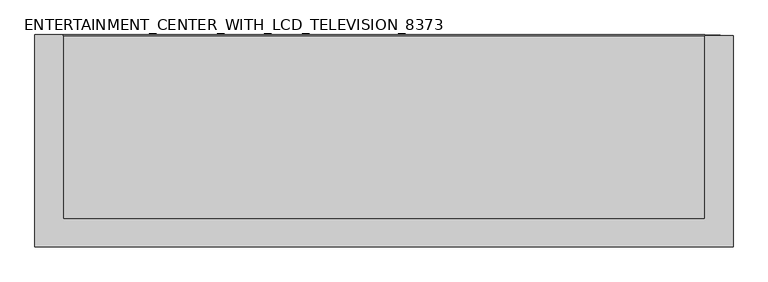
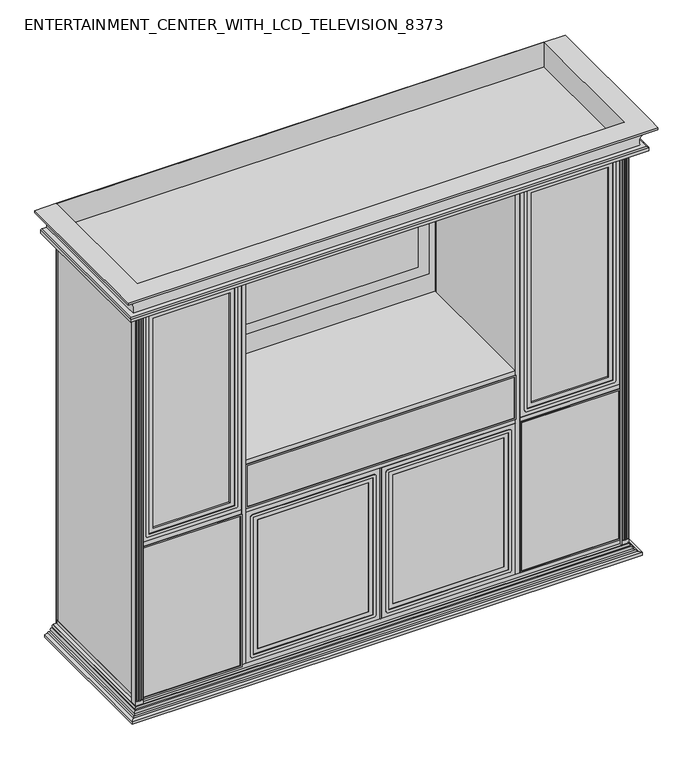
"""IFC4 building model written with IfcOpenShell, lengths in millimetres: furniture geometry, ENTERTAINMENT_CENTER_WITH_LCD_TELEVISION_8373."""

from ifc_helpers import new_model, si_unit, point, frame, frame_2d, origin, origin_with_axes, place, context, project, spatial, polyline, circle_curve, ellipse_curve, trimmed, segment, composite_curve, outline, extrude, faceted_brep, source, transform, mapped, element, save
from ifc_brep_helpers import plane_surface, cylinder_surface, revolved_surface, advanced_brep


def entertainment_center_with_lcd_television_8373_4fd72ac7(model_context):
    return source(origin(), model_context, "Body", "SolidModel", [
        extrude(outline(polyline([(-1066.8, -9.525), (-1066.8, 0.0), (-1047.75, 0.0), (-1047.75, -9.525), (-1047.75, -609.6), (-1066.8, -609.6), (-1066.8, -9.525)])), frame((0.0, 0.0, 19.05), z_axis=(0.0, 0.0, 1.0), x_axis=(1.0, 0.0, 0.0)), (0.0, 0.0, 1.0), 1790.7),
        extrude(outline(polyline([(1066.8, -9.525), (1066.8, -609.6), (1047.75, -609.6), (1047.75, -9.525), (1047.75, 0.0), (1066.8, 0.0), (1066.8, -9.525)])), frame((0.0, 0.0, 19.05), z_axis=(0.0, 0.0, 1.0), x_axis=(1.0, 0.0, 0.0)), (0.0, 0.0, 1.0), 1790.7),
        extrude(outline(polyline([(609.6, -9.525), (609.6, -609.6), (590.55, -609.6), (590.55, -9.525), (590.55, 0.0), (609.6, 0.0), (609.6, -9.525)])), frame((0.0, 0.0, 19.05), z_axis=(0.0, 0.0, 1.0), x_axis=(1.0, 0.0, 0.0)), (0.0, 0.0, 1.0), 1790.7),
        extrude(outline(polyline([(-590.55, -9.525), (-590.55, -609.6), (-609.6, -609.6), (-609.6, -9.525), (-609.6, 0.0), (-590.55, 0.0), (-590.55, -9.525)])), frame((0.0, 0.0, 19.05), z_axis=(0.0, 0.0, 1.0), x_axis=(1.0, 0.0, 0.0)), (0.0, 0.0, 1.0), 1790.7),
        extrude(outline(polyline([(590.55, -609.6), (-590.55, -609.6), (-590.55, 0.0), (590.55, 0.0), (590.55, -609.6)])), frame((0.0, 0.0, 717.55), z_axis=(0.0, 0.0, 1.0), x_axis=(1.0, 0.0, 0.0)), (0.0, 0.0, 1.0), 19.05),
        extrude(outline(polyline([(2.2792992, -609.6), (-2.4300659, -609.6), (-2.4300659, -590.55), (2.2792992, -590.55), (2.2792992, -609.6)])), frame((0.0, 0.0, 19.05), z_axis=(0.0, 0.0, 1.0), x_axis=(1.0, 0.0, 0.0)), (0.0, 0.0, 1.0), 698.5),
        extrude(outline(polyline([(717.55, -3.175), (717.55, -590.55), (19.05, -590.55), (19.05, -3.175), (717.55, -3.175)]), holes=[polyline([(666.75, -53.975), (69.85, -53.975), (69.85, -539.75), (666.75, -539.75), (666.75, -53.975)])]), frame((0.0, -609.6, 0.0), z_axis=(0.0, 1.0, 0.0), x_axis=(0.0, 0.0, 1.0)), (0.0, 0.0, 1.0), 19.05),
        extrude(outline(polyline([(717.55, 590.55), (717.55, 3.175), (19.05, 3.175), (19.05, 590.55), (717.55, 590.55)]), holes=[polyline([(666.75, 539.75), (69.85, 539.75), (69.85, 53.975), (666.75, 53.975), (666.75, 539.75)])]), frame((0.0, -609.6, 0.0), z_axis=(0.0, 1.0, 0.0), x_axis=(0.0, 0.0, 1.0)), (0.0, 0.0, 1.0), 19.05),
        extrude(outline(polyline([(-53.975, -609.6), (-539.75, -609.6), (-539.75, -606.425), (-53.975, -606.425), (-53.975, -609.6)])), frame((0.0, 0.0, 69.85), z_axis=(0.0, 0.0, 1.0), x_axis=(1.0, 0.0, 0.0)), (0.0, 0.0, 1.0), 596.9),
        extrude(outline(polyline([(539.75, -609.6), (53.975, -609.6), (53.975, -606.425), (539.75, -606.425), (539.75, -609.6)])), frame((0.0, 0.0, 69.85), z_axis=(0.0, 0.0, 1.0), x_axis=(1.0, 0.0, 0.0)), (0.0, 0.0, 1.0), 596.9),
        extrude(outline(polyline([(-609.6, -609.6), (-1047.75, -609.6), (-1047.75, 0.0), (-609.6, 0.0), (-609.6, -609.6)])), frame((0.0, 0.0, 717.55), z_axis=(0.0, 0.0, 1.0), x_axis=(1.0, 0.0, 0.0)), (0.0, 0.0, 1.0), 19.05),
        extrude(outline(polyline([(1047.75, -609.6), (609.6, -609.6), (609.6, 0.0), (1047.75, 0.0), (1047.75, -609.6)])), frame((0.0, 0.0, 717.55), z_axis=(0.0, 0.0, 1.0), x_axis=(1.0, 0.0, 0.0)), (0.0, 0.0, 1.0), 19.05),
        extrude(outline(polyline([(590.55, -609.6), (-590.55, -609.6), (-590.55, 0.0), (590.55, 0.0), (590.55, -609.6)])), frame((0.0, 0.0, 939.8), z_axis=(0.0, 0.0, 1.0), x_axis=(1.0, 0.0, 0.0)), (0.0, 0.0, 1.0), 19.05),
        extrude(outline(polyline([(590.55, -609.6), (-590.55, -609.6), (-590.55, -590.55), (590.55, -590.55), (590.55, -609.6)])), frame((0.0, 0.0, 736.6), z_axis=(0.0, 0.0, 1.0), x_axis=(1.0, 0.0, 0.0)), (0.0, 0.0, 1.0), 203.2),
        extrude(outline(polyline([(-609.6, -609.6), (-1047.75, -609.6), (-1047.75, -590.55), (-609.6, -590.55), (-609.6, -609.6)])), frame((0.0, 0.0, 19.05), z_axis=(0.0, 0.0, 1.0), x_axis=(1.0, 0.0, 0.0)), (0.0, 0.0, 1.0), 698.5),
        extrude(outline(polyline([(1047.75, -609.6), (609.6, -609.6), (609.6, -590.55), (1047.75, -590.55), (1047.75, -609.6)])), frame((0.0, 0.0, 19.05), z_axis=(0.0, 0.0, 1.0), x_axis=(1.0, 0.0, 0.0)), (0.0, 0.0, 1.0), 698.5),
        extrude(outline(polyline([(-609.6, -547.2385418), (-1047.75, -547.2385418), (-1047.75, 0.0), (-609.6, 0.0), (-609.6, -547.2385418)])), frame((0.0, 0.0, 1291.7854241), z_axis=(0.0, 0.0, 1.0), x_axis=(1.0, 0.0, 0.0)), (0.0, 0.0, 1.0), 3.175),
        extrude(outline(polyline([(1047.75, -547.2385418), (609.6, -547.2385418), (609.6, 0.0), (1047.75, 0.0), (1047.75, -547.2385418)])), frame((0.0, 0.0, 1291.7854241), z_axis=(0.0, 0.0, 1.0), x_axis=(1.0, 0.0, 0.0)), (0.0, 0.0, 1.0), 3.175),
        extrude(outline(polyline([(-609.6, -547.2385418), (-1047.75, -547.2385418), (-1047.75, 0.0), (-609.6, 0.0), (-609.6, -547.2385418)])), frame((0.0, 0.0, 887.1114077), z_axis=(0.0, 0.0, 1.0), x_axis=(1.0, 0.0, 0.0)), (0.0, 0.0, 1.0), 3.175),
        extrude(outline(polyline([(1047.75, -547.2385418), (609.6, -547.2385418), (609.6, 0.0), (1047.75, 0.0), (1047.75, -547.2385418)])), frame((0.0, 0.0, 887.1114077), z_axis=(0.0, 0.0, 1.0), x_axis=(1.0, 0.0, 0.0)), (0.0, 0.0, 1.0), 3.175),
        extrude(outline(polyline([(-609.6, -547.2385418), (-1047.75, -547.2385418), (-1047.75, 0.0), (-609.6, 0.0), (-609.6, -547.2385418)])), frame((0.0, 0.0, 1501.775), z_axis=(0.0, 0.0, 1.0), x_axis=(1.0, 0.0, 0.0)), (0.0, 0.0, 1.0), 3.175),
        extrude(outline(polyline([(1047.75, -547.2385418), (609.6, -547.2385418), (609.6, 0.0), (1047.75, 0.0), (1047.75, -547.2385418)])), frame((0.0, 0.0, 1501.775), z_axis=(0.0, 0.0, 1.0), x_axis=(1.0, 0.0, 0.0)), (0.0, 0.0, 1.0), 3.175),
        extrude(outline(polyline([(546.1, -29.8156633), (-546.1, -29.8156633), (-546.1, 0.0), (546.1, 0.0), (546.1, -29.8156633)])), frame((0.0, 0.0, 1073.15), z_axis=(0.0, 0.0, 1.0), x_axis=(1.0, 0.0, 0.0)), (0.0, 0.0, 1.0), 660.4),
        extrude(outline(polyline([(495.3, -36.468697), (-495.3, -36.468697), (-495.3, -29.8156633), (495.3, -29.8156633), (495.3, -36.468697)])), frame((0.0, 0.0, 1123.95), z_axis=(0.0, 0.0, 1.0), x_axis=(1.0, 0.0, 0.0)), (0.0, 0.0, 1.0), 558.8),
        extrude(outline(polyline([(1066.8, 3.175), (1066.8, 0.0), (-1066.8, 0.0), (-1066.8, 3.175), (1066.8, 3.175)])), origin_with_axes(), (0.0, 0.0, 1.0), 1942.4645734),
        extrude(outline(polyline([(1066.8, -609.6), (-1066.8, -609.6), (-1066.8, 0.0), (1066.8, 0.0), (1066.8, -609.6)])), origin_with_axes(), (0.0, 0.0, 1.0), 19.05),
        extrude(outline(polyline([(1066.8, -609.6), (-1066.8, -609.6), (-1066.8, 0.0), (1066.8, 0.0), (1066.8, -609.6)])), frame((0.0, 0.0, 1809.75), z_axis=(0.0, 0.0, 1.0), x_axis=(1.0, 0.0, 0.0)), (0.0, 0.0, 1.0), 19.05),
        advanced_brep(
        [(1066.8, 3.175, 0.0), (1066.8, -609.6, 0.0), (-1066.8, -609.6, 0.0), (-1066.8, 3.175, 0.0), (-1079.6325221, 3.175, 0.0), (-1079.6325221, -622.4325221, 0.0), (1079.6325221, -622.4325221, 0.0), (1079.6325221, 3.175, 0.0), (-1066.8, 3.175, -47.0950188), (-1066.8, -609.6, -47.0950188), (1066.8, -609.6, -47.0950188), (1066.8, 3.175, -47.0950188), (1117.6, 3.175, -47.0950188), (1117.6, -660.4, -47.0950188), (-1117.6, -660.4, -47.0950188), (-1117.6, 3.175, -47.0950188), (-1117.6, 3.175, -34.925), (-1103.8793251, 3.175, -32.3686785), (-1097.6139898, 3.175, -29.2621608), (-1090.9923514, 3.175, -24.0948191), (-1084.548346, 3.175, -15.7775241), (-1082.539262, 3.175, -11.7365609), (-1079.9769539, 3.175, -2.8346923), (-1117.6, -660.4, -34.925), (1117.6, -660.4, -34.925), (1117.6, 3.175, -34.925), (1079.9769539, 3.175, -2.8346923), (1082.539262, 3.175, -11.7365609), (1084.548346, 3.175, -15.7775241), (1090.9923514, 3.175, -24.0948191), (1097.6139898, 3.175, -29.2621608), (1103.8793251, 3.175, -32.3686785), (1079.9769539, -622.7769539, -2.8346923), (-1079.9769539, -622.7769539, -2.8346923), (1103.8793251, -646.6793251, -32.3686785), (1097.6139898, -640.4139898, -29.2621608), (1090.9923514, -633.7923514, -24.0948191), (1084.548346, -627.348346, -15.7775241), (1082.539262, -625.339262, -11.7365609), (-1103.8793251, -646.6793251, -32.3686785), (-1097.6139898, -640.4139898, -29.2621608), (-1090.9923514, -633.7923514, -24.0948191), (-1084.548346, -627.348346, -15.7775241), (-1082.539262, -625.339262, -11.7365609)],
        [
            (0, 1),
            (1, 2),
            (2, 3),
            (3, 4),
            (4, 5),
            (5, 6),
            (6, 7),
            (7, 0),
            (8, 9),
            (9, 10),
            (10, 11),
            (11, 12),
            (12, 13),
            (13, 14),
            (14, 15),
            (15, 8),
            (15, 16),
            (16, 17, circle_curve(frame((-1117.6, 3.175, 3.175), z_axis=(0.0, -1.0, 0.0), x_axis=(1.0, 0.0, 0.0)), 38.1)),
            (17, 18, circle_curve(frame((-1100.6752321, 3.175, -30.9594728), z_axis=(0.0, 1.0, 0.0), x_axis=(1.0, 0.0, 0.0)), 3.5002961)),
            (18, 19, circle_curve(frame((-1117.6, 3.175, 3.175), z_axis=(0.0, -1.0, 0.0), x_axis=(1.0, 0.0, 0.0)), 38.1)),
            (19, 20, circle_curve(frame((-1087.4818585, 3.175, -20.1596857), z_axis=(0.0, 1.0, 0.0), x_axis=(1.0, 0.0, 0.0)), 5.2734083)),
            (20, 21, circle_curve(frame((-1117.6, 3.175, 3.175), z_axis=(0.0, -1.0, 0.0), x_axis=(1.0, 0.0, 0.0)), 38.1)),
            (21, 22, circle_curve(frame((-1080.9865607, 3.175, -7.3637886), z_axis=(0.0, 1.0, 0.0), x_axis=(1.0, 0.0, 0.0)), 4.6402607)),
            (22, 4, circle_curve(frame((-1117.6, 3.175, 3.175), z_axis=(0.0, -1.0, 0.0), x_axis=(1.0, 0.0, 0.0)), 38.1)),
            (3, 8),
            (14, 23),
            (23, 16),
            (13, 24),
            (24, 23),
            (12, 25),
            (25, 24),
            (11, 0),
            (7, 26, circle_curve(frame((1117.6, 3.175, 3.175), z_axis=(0.0, -1.0, 0.0), x_axis=(-1.0, 0.0, 0.0)), 38.1)),
            (26, 27, circle_curve(frame((1080.9865607, 3.175, -7.3637886), z_axis=(0.0, 1.0, 0.0), x_axis=(-1.0, 0.0, 0.0)), 4.6402607)),
            (27, 28, circle_curve(frame((1117.6, 3.175, 3.175), z_axis=(0.0, -1.0, 0.0), x_axis=(-1.0, 0.0, 0.0)), 38.1)),
            (28, 29, circle_curve(frame((1087.4818585, 3.175, -20.1596857), z_axis=(0.0, 1.0, 0.0), x_axis=(-1.0, 0.0, 0.0)), 5.2734083)),
            (29, 30, circle_curve(frame((1117.6, 3.175, 3.175), z_axis=(0.0, -1.0, 0.0), x_axis=(-1.0, 0.0, 0.0)), 38.1)),
            (30, 31, circle_curve(frame((1100.6752321, 3.175, -30.9594728), z_axis=(0.0, 1.0, 0.0), x_axis=(-1.0, 0.0, 0.0)), 3.5002961)),
            (31, 25, circle_curve(frame((1117.6, 3.175, 3.175), z_axis=(0.0, -1.0, 0.0), x_axis=(-1.0, 0.0, 0.0)), 38.1)),
            (10, 1),
            (9, 2),
            (32, 26),
            (6, 32, ellipse_curve(frame((1117.6, -660.4, 3.175), z_axis=(-0.7071067811865475, -0.7071067811865476, 0.0), x_axis=(-0.7071067811865475, 0.7071067811865475, 0.0)), 53.8815367, 38.1)),
            (33, 32),
            (5, 33, ellipse_curve(frame((-1117.6, -660.4, 3.175), z_axis=(-0.7071067811865476, 0.7071067811865475, 0.0), x_axis=(0.7071067811865475, 0.7071067811865475, 0.0)), 53.8815367, 38.1)),
            (22, 33),
            (31, 34),
            (34, 24, ellipse_curve(frame((1117.6, -660.4, 3.175), z_axis=(-0.7071067811865475, -0.7071067811865476, 0.0), x_axis=(-0.7071067811865475, 0.7071067811865475, 0.0)), 53.8815367, 38.1)),
            (30, 35),
            (35, 34, ellipse_curve(frame((1100.6752321, -643.4752321, -30.9594728), z_axis=(0.7071067811865475, 0.7071067811865476, 0.0), x_axis=(0.7071067811865475, -0.7071067811865475, 0.0)), 4.9501661, 3.5002961)),
            (29, 36),
            (36, 35, ellipse_curve(frame((1117.6, -660.4, 3.175), z_axis=(-0.7071067811865475, -0.7071067811865476, 0.0), x_axis=(-0.7071067811865475, 0.7071067811865475, 0.0)), 53.8815367, 38.1)),
            (28, 37),
            (37, 36, ellipse_curve(frame((1087.4818585, -630.2818585, -20.1596857), z_axis=(0.7071067811865475, 0.7071067811865476, 0.0), x_axis=(0.7071067811865475, -0.7071067811865475, 0.0)), 7.4577256, 5.2734083)),
            (27, 38),
            (38, 37, ellipse_curve(frame((1117.6, -660.4, 3.175), z_axis=(-0.7071067811865475, -0.7071067811865476, 0.0), x_axis=(-0.7071067811865475, 0.7071067811865475, 0.0)), 53.8815367, 38.1)),
            (32, 38, ellipse_curve(frame((1080.9865607, -623.7865607, -7.3637886), z_axis=(0.7071067811865475, 0.7071067811865476, 0.0), x_axis=(0.7071067811865475, -0.7071067811865475, 0.0)), 6.5623196, 4.6402607)),
            (34, 39),
            (39, 23, ellipse_curve(frame((-1117.6, -660.4, 3.175), z_axis=(-0.7071067811865476, 0.7071067811865475, 0.0), x_axis=(0.7071067811865475, 0.7071067811865475, 0.0)), 53.8815367, 38.1)),
            (35, 40),
            (40, 39, ellipse_curve(frame((-1100.6752321, -643.4752321, -30.9594728), z_axis=(0.7071067811865476, -0.7071067811865475, 0.0), x_axis=(-0.7071067811865475, -0.7071067811865475, 0.0)), 4.9501661, 3.5002961)),
            (36, 41),
            (41, 40, ellipse_curve(frame((-1117.6, -660.4, 3.175), z_axis=(-0.7071067811865476, 0.7071067811865475, 0.0), x_axis=(0.7071067811865475, 0.7071067811865475, 0.0)), 53.8815367, 38.1)),
            (37, 42),
            (42, 41, ellipse_curve(frame((-1087.4818585, -630.2818585, -20.1596857), z_axis=(0.7071067811865476, -0.7071067811865475, 0.0), x_axis=(-0.7071067811865475, -0.7071067811865475, 0.0)), 7.4577256, 5.2734083)),
            (38, 43),
            (43, 42, ellipse_curve(frame((-1117.6, -660.4, 3.175), z_axis=(-0.7071067811865476, 0.7071067811865475, 0.0), x_axis=(0.7071067811865475, 0.7071067811865475, 0.0)), 53.8815367, 38.1)),
            (33, 43, ellipse_curve(frame((-1080.9865607, -623.7865607, -7.3637886), z_axis=(0.7071067811865476, -0.7071067811865475, 0.0), x_axis=(-0.7071067811865475, -0.7071067811865475, 0.0)), 6.5623196, 4.6402607)),
            (39, 17),
            (40, 18),
            (41, 19),
            (42, 20),
            (43, 21),
        ],
        [
            plane_surface(frame((-1117.6, 3.175, 0.0), z_axis=(0.0, 0.0, 1.0), x_axis=(-1.0, 0.0, 0.0))),
            plane_surface(frame((-1117.6, 3.175, -47.0950188), z_axis=(0.0, 0.0, -1.0), x_axis=(1.0, 0.0, 0.0))),
            plane_surface(frame((-1066.8, 3.175, 0.0), z_axis=(0.0, 1.0, 0.0), x_axis=(0.0, 0.0, -1.0))),
            plane_surface(frame((-1117.6, 3.175, 0.0), z_axis=(-1.0, 0.0, 0.0), x_axis=(0.0, 0.0, -1.0))),
            plane_surface(frame((-1117.6, -660.4, 0.0), z_axis=(0.0, -1.0, 0.0), x_axis=(0.0, 0.0, -1.0))),
            plane_surface(frame((1117.6, -660.4, 0.0), z_axis=(1.0, 0.0, 0.0), x_axis=(0.0, 0.0, -1.0))),
            plane_surface(frame((1117.6, 3.175, 0.0), z_axis=(0.0, 1.0, 0.0), x_axis=(0.0, 0.0, -1.0))),
            plane_surface(frame((1066.8, 3.175, 0.0), z_axis=(-1.0, 0.0, 0.0), x_axis=(0.0, 0.0, -1.0))),
            plane_surface(frame((1066.8, -609.6, 0.0), z_axis=(0.0, 1.0, 0.0), x_axis=(0.0, 0.0, -1.0))),
            plane_surface(frame((-1066.8, -609.6, 0.0), z_axis=(1.0, 0.0, 0.0), x_axis=(0.0, 0.0, -1.0))),
            revolved_surface(polyline([(1079.5, 3.175, 3.175), (1079.5, -698.4999999813218, 3.175)]), (1117.6, 3.175, 3.175), (0.0, 1.0, 0.0)),
            revolved_surface(polyline([(1155.6999999813218, -622.3, 3.175), (-1155.6999999813215, -622.3, 3.175)]), (1117.6, -660.4, 3.175), (1.0, 0.0, 0.0)),
            revolved_surface(polyline([(-1079.5, -698.4999999813218, 3.175), (-1079.5, 3.1749999999999545, 3.175)]), (-1117.6, -660.4, 3.175), (0.0, -1.0, 0.0)),
            cylinder_surface(frame((1100.6752321, 3.175, -30.9594728), z_axis=(0.0, -1.0, 0.0), x_axis=(-1.0, 0.0, 0.0)), 3.5002961),
            cylinder_surface(frame((1087.4818585, 3.175, -20.1596857), z_axis=(0.0, -1.0, 0.0), x_axis=(-1.0, 0.0, 0.0)), 5.2734083),
            cylinder_surface(frame((1080.9865607, 3.175, -7.3637886), z_axis=(0.0, -1.0, 0.0), x_axis=(-1.0, 0.0, 0.0)), 4.6402607),
            cylinder_surface(frame((1117.6, -643.4752321, -30.9594728), z_axis=(-1.0, 0.0, 0.0), x_axis=(0.0, 1.0, 0.0)), 3.5002961),
            cylinder_surface(frame((1117.6, -630.2818585, -20.1596857), z_axis=(-1.0, 0.0, 0.0), x_axis=(0.0, 1.0, 0.0)), 5.2734083),
            cylinder_surface(frame((1117.6, -623.7865607, -7.3637886), z_axis=(-1.0, 0.0, 0.0), x_axis=(0.0, 1.0, 0.0)), 4.6402607),
            cylinder_surface(frame((-1100.6752321, -660.4, -30.9594728), z_axis=(0.0, 1.0, 0.0), x_axis=(1.0, 0.0, 0.0)), 3.5002961),
            cylinder_surface(frame((-1087.4818585, -660.4, -20.1596857), z_axis=(0.0, 1.0, 0.0), x_axis=(1.0, 0.0, 0.0)), 5.2734083),
            cylinder_surface(frame((-1080.9865607, -660.4, -7.3637886), z_axis=(0.0, 1.0, 0.0), x_axis=(1.0, 0.0, 0.0)), 4.6402607),
        ],
        [
            (0, [[1, 2, 3, 4, 5, 6, 7, 8]]),
            (1, [[9, 10, 11, 12, 13, 14, 15, 16]]),
            (2, [[-16, 17, 18, 19, 20, 21, 22, 23, 24, -4, 25]]),
            (3, [[-15, 26, 27, -17]]),
            (4, [[-14, 28, 29, -26]]),
            (5, [[-13, 30, 31, -28]]),
            (6, [[-12, 32, -8, 33, 34, 35, 36, 37, 38, 39, -30]]),
            (7, [[-1, -32, -11, 40]]),
            (8, [[-2, -40, -10, 41]]),
            (9, [[-3, -41, -9, -25]]),
            (10, [[42, -33, -7, 43]]),
            (11, [[44, -43, -6, 45]]),
            (12, [[46, -45, -5, -24]]),
            (10, [[47, 48, -31, -39]]),
            (13, [[-47, -38, 49, 50]]),
            (10, [[-49, -37, 51, 52]]),
            (14, [[-51, -36, 53, 54]]),
            (10, [[-53, -35, 55, 56]]),
            (15, [[-42, 57, -55, -34]]),
            (11, [[-48, 58, 59, -29]]),
            (16, [[-50, 60, 61, -58]]),
            (11, [[-52, 62, 63, -60]]),
            (17, [[-54, 64, 65, -62]]),
            (11, [[-56, 66, 67, -64]]),
            (18, [[-44, 68, -66, -57]]),
            (12, [[-59, 69, -18, -27]]),
            (19, [[-61, 70, -19, -69]]),
            (12, [[-63, 71, -20, -70]]),
            (20, [[-65, 72, -21, -71]]),
            (12, [[-67, 73, -22, -72]]),
            (21, [[-46, -23, -73, -68]]),
        ],
    ),
        extrude(outline(polyline([(1809.75, -609.6), (1809.75, -1047.75), (736.6, -1047.75), (736.6, -609.6), (1809.75, -609.6)]), holes=[polyline([(1758.95, -660.4), (787.4, -660.4), (787.4, -996.95), (1758.95, -996.95), (1758.95, -660.4)])]), frame((0.0, -609.6, 0.0), z_axis=(0.0, 1.0, 0.0), x_axis=(0.0, 0.0, 1.0)), (0.0, 0.0, 1.0), 19.05),
        extrude(outline(polyline([(1809.75, 1047.75), (1809.75, 609.6), (736.6, 609.6), (736.6, 1047.75), (1809.75, 1047.75)]), holes=[polyline([(1758.95, 996.95), (787.4, 996.95), (787.4, 660.4), (1758.95, 660.4), (1758.95, 996.95)])]), frame((0.0, -609.6, 0.0), z_axis=(0.0, 1.0, 0.0), x_axis=(0.0, 0.0, 1.0)), (0.0, 0.0, 1.0), 19.05),
        extrude(outline(polyline([(-996.95, -596.9), (-660.4, -596.9), (-660.4, -603.25), (-996.95, -603.25), (-996.95, -596.9)])), frame((0.0, 0.0, 787.4), z_axis=(0.0, 0.0, 1.0), x_axis=(1.0, 0.0, 0.0)), (0.0, 0.0, 1.0), 971.55),
        extrude(outline(polyline([(660.4, -596.9), (996.95, -596.9), (996.95, -603.25), (660.4, -603.25), (660.4, -596.9)])), frame((0.0, 0.0, 787.4), z_axis=(0.0, 0.0, 1.0), x_axis=(1.0, 0.0, 0.0)), (0.0, 0.0, 1.0), 971.55),
        faceted_brep([(-1079.6325221, -590.55, 1828.8), (-1047.4045021, -590.55, 1828.8), (-1047.4045021, -590.55, -1.5875), (-1079.6325221, -590.55, -1.5875), (-1079.6325221, -622.4325221, 1828.8), (-1079.6325221, -622.4325221, -1.5875), (-1047.4045021, -622.4325221, -1.5875), (-1047.4045021, -622.4325221, 1828.8), (-1075.7590463, -622.4325221, 1790.7), (-1069.4090463, -622.4325221, 1790.7), (-1069.4090463, -622.4325221, 19.05), (-1075.7590463, -622.4325221, 19.05), (-1065.6299087, -622.4325221, 1790.7), (-1059.4693889, -622.4325221, 1790.7), (-1059.4693889, -622.4325221, 19.05), (-1065.6299087, -622.4325221, 19.05), (-1056.2121026, -622.4325221, 1790.7), (-1050.4764463, -622.4325221, 1790.7), (-1050.4764463, -622.4325221, 19.05), (-1056.2121026, -622.4325221, 19.05), (-1075.7590463, -613.965625, 1790.7), (-1069.4090463, -613.965625, 1790.7), (-1065.6299087, -613.965625, 1790.7), (-1059.4693889, -613.965625, 1790.7), (-1056.2121026, -613.965625, 1790.7), (-1050.4764463, -613.965625, 1790.7), (-1069.4090463, -613.965625, 19.05), (-1075.7590463, -613.965625, 19.05), (-1059.4693889, -613.965625, 19.05), (-1065.6299087, -613.965625, 19.05), (-1050.4764463, -613.965625, 19.05), (-1056.2121026, -613.965625, 19.05)], [[[0, 1, 2, 3]], [[4, 5, 6, 7], [8, 9, 10, 11], [12, 13, 14, 15], [16, 17, 18, 19]], [[1, 0, 4, 7]], [[2, 1, 7, 6]], [[3, 2, 6, 5]], [[0, 3, 5, 4]], [[8, 20, 21, 9]], [[12, 22, 23, 13]], [[16, 24, 25, 17]], [[10, 26, 27, 11]], [[14, 28, 29, 15]], [[18, 30, 31, 19]], [[9, 21, 26, 10]], [[21, 20, 27, 26]], [[20, 8, 11, 27]], [[13, 23, 28, 14]], [[23, 22, 29, 28]], [[22, 12, 15, 29]], [[17, 25, 30, 18]], [[25, 24, 31, 30]], [[24, 16, 19, 31]]]),
        faceted_brep([(1079.6325221, -590.55, 1828.8), (1079.6325221, -590.55, -1.5875), (1048.0954979, -590.55, -1.5875), (1048.0954979, -590.55, 1828.8), (1079.6325221, -622.4325221, 1828.8), (1048.0954979, -622.4325221, 1828.8), (1048.0954979, -622.4325221, -1.5875), (1079.6325221, -622.4325221, -1.5875), (1051.3396559, -622.4325221, 1790.7), (1057.2927809, -622.4325221, 1790.7), (1057.2927809, -622.4325221, 19.05), (1051.3396559, -622.4325221, 19.05), (1061.7755941, -622.4325221, 1790.7), (1066.8, -622.4325221, 1790.7), (1066.8, -622.4325221, 19.05), (1061.7755941, -622.4325221, 19.05), (1070.6337288, -622.4325221, 1790.7), (1076.6647367, -622.4325221, 1790.7), (1076.6647367, -622.4325221, 19.05), (1070.6337288, -622.4325221, 19.05), (1051.3396559, -614.4052284, 1790.7), (1057.2927809, -614.4052284, 1790.7), (1061.7755941, -614.6127689, 1790.7), (1066.8, -614.6127689, 1790.7), (1070.6337288, -614.4420648, 1790.7), (1076.6647367, -614.4420648, 1790.7), (1051.3396559, -614.4052284, 19.05), (1057.2927809, -614.4052284, 19.05), (1061.7755941, -614.6127689, 19.05), (1066.8, -614.6127689, 19.05), (1076.6647367, -614.4420648, 19.05), (1070.6337288, -614.4420648, 19.05)], [[[0, 1, 2, 3]], [[4, 5, 6, 7], [8, 9, 10, 11], [12, 13, 14, 15], [16, 17, 18, 19]], [[1, 0, 4, 7]], [[2, 1, 7, 6]], [[3, 2, 6, 5]], [[0, 3, 5, 4]], [[20, 21, 9, 8]], [[22, 23, 13, 12]], [[16, 24, 25, 17]], [[26, 11, 10, 27]], [[28, 15, 14, 29]], [[18, 30, 31, 19]], [[20, 8, 11, 26]], [[9, 21, 27, 10]], [[21, 20, 26, 27]], [[22, 12, 15, 28]], [[13, 23, 29, 14]], [[23, 22, 28, 29]], [[24, 16, 19, 31]], [[25, 24, 31, 30]], [[17, 25, 30, 18]]]),
        extrude(outline(composite_curve([segment(polyline([(1784.35, -1028.6298662), (762.0, -1028.6298662)]), True, "CONTINUOUS"), segment(trimmed(circle_curve(frame_2d((762.0, -1022.2798662)), 6.35), [point((762.0, -1028.6298662))], [point((755.65, -1022.2798662))], False, "CARTESIAN"), True, "CONTINUOUS"), segment(polyline([(755.65, -1022.2798662), (755.65, -634.9298662)]), True, "CONTINUOUS"), segment(trimmed(circle_curve(frame_2d((762.0, -634.9298662)), 6.35), [point((755.65, -634.9298662))], [point((762.0, -628.5798662))], False, "CARTESIAN"), True, "CONTINUOUS"), segment(polyline([(762.0, -628.5798662), (1784.35, -628.5798662)]), True, "CONTINUOUS"), segment(trimmed(circle_curve(frame_2d((1784.35, -634.9298662)), 6.35), [point((1784.35, -628.5798662))], [point((1790.7, -634.9298662))], False, "CARTESIAN"), True, "CONTINUOUS"), segment(polyline([(1790.7, -634.9298662), (1790.7, -1022.2798662)]), True, "CONTINUOUS"), segment(trimmed(circle_curve(frame_2d((1784.35, -1022.2798662)), 6.35), [point((1790.7, -1022.2798662))], [point((1784.35, -1028.6298662))], False, "CARTESIAN"), True, "CONTINUOUS")], self_intersect=False), holes=[polyline([(768.35, -1015.9298662), (1778.0, -1015.9298662), (1778.0, -641.2798662), (768.35, -641.2798662), (768.35, -1015.9298662)])]), frame((0.0, -612.775, 0.0), z_axis=(0.0, 1.0, 0.0), x_axis=(0.0, 0.0, 1.0)), (0.0, 0.0, 1.0), 3.175),
        advanced_brep(
        [(-1066.8, 3.175, 1942.4645734), (-1160.5617187, 3.175, 1942.4645734), (-1160.5617187, -703.3617187, 1942.4645734), (1160.5617187, -703.3617187, 1942.4645734), (1160.5617187, -640.3503235, 1942.4645734), (1160.5617187, 0.0, 1942.4645734), (1066.8, 0.0, 1942.4645734), (1066.8, -609.6, 1942.4645734), (-1066.8, -609.6, 1942.4645734), (-1066.8, 3.175, 1828.8), (-1066.8, -609.6, 1828.8), (1066.8, -609.6, 1828.8), (1066.8, 0.0, 1828.8), (1135.1617187, 0.0, 1828.8), (1135.1617187, -677.9617187, 1828.8), (-1135.1617187, -677.9617187, 1828.8), (-1135.1617187, 3.175, 1828.8), (-1135.1617187, 3.175, 1841.5), (-1128.8117187, 3.175, 1847.85), (-1109.7617187, 3.175, 1847.85), (-1160.5617187, 3.175, 1931.9038907), (-1160.5617187, -703.3617187, 1931.9038907), (1160.5617187, -703.3617187, 1931.9038907), (1160.5617187, -640.3503235, 1931.9038907), (1160.5617187, 0.0, 1931.9038907), (1109.7617187, 0.0, 1847.85), (1128.8117187, 0.0, 1847.85), (1135.1617187, 0.0, 1841.5), (1109.7617187, -640.3503235, 1847.85), (1109.7617187, -652.5617187, 1847.85), (-1109.7617187, -652.5617187, 1847.85), (-1128.8117187, -671.6117187, 1847.85), (1128.8117187, -671.6117187, 1847.85), (1128.8117187, -640.3503235, 1847.85), (1135.1617187, -640.3503235, 1841.5), (1135.1617187, -677.9617187, 1841.5), (-1135.1617187, -677.9617187, 1841.5)],
        [
            (0, 1),
            (1, 2),
            (2, 3),
            (3, 4),
            (4, 5),
            (5, 6),
            (6, 7),
            (7, 8),
            (8, 0),
            (9, 10),
            (10, 11),
            (11, 12),
            (12, 13),
            (13, 14),
            (14, 15),
            (15, 16),
            (16, 9),
            (0, 9),
            (16, 17),
            (17, 18, circle_curve(frame((-1128.8117187, 3.175, 1841.5), z_axis=(0.0, 1.0, 0.0), x_axis=(1.0, 0.0, 0.0)), 6.35)),
            (18, 19),
            (19, 20, circle_curve(frame((-1180.3298192, 3.175, 1862.5785123), z_axis=(0.0, -1.0, 0.0), x_axis=(1.0, 0.0, 0.0)), 72.0887362)),
            (20, 1),
            (20, 21),
            (21, 2),
            (21, 22),
            (22, 3),
            (22, 23),
            (23, 4),
            (23, 24),
            (24, 5),
            (24, 25, circle_curve(frame((1180.3298192, 0.0, 1862.5785123), z_axis=(0.0, -1.0, 0.0), x_axis=(-1.0, 0.0, 0.0)), 72.0887362)),
            (25, 26),
            (26, 27, circle_curve(frame((1128.8117187, 0.0, 1841.5), z_axis=(0.0, 1.0, 0.0), x_axis=(-1.0, 0.0, 0.0)), 6.35)),
            (27, 13),
            (12, 6),
            (11, 7),
            (10, 8),
            (25, 28),
            (28, 29),
            (29, 30),
            (30, 19),
            (18, 31),
            (31, 32),
            (32, 33),
            (33, 26),
            (23, 28, circle_curve(frame((1180.3298192, -640.3503235, 1862.5785123), z_axis=(0.0, -1.0, 0.0), x_axis=(-1.0, 0.0, 0.0)), 72.0887362)),
            (22, 29, ellipse_curve(frame((1180.3298192, -723.1298192, 1862.5785123), z_axis=(-0.7071067811865475, -0.7071067811865475, 0.0), x_axis=(-0.7071067811865474, 0.7071067811865476, 0.0)), 101.9488684, 72.0887362)),
            (21, 30, ellipse_curve(frame((-1180.3298192, -723.1298192, 1862.5785123), z_axis=(-0.7071067811865475, 0.7071067811865475, 0.0), x_axis=(0.7071067811865476, 0.7071067811865474, 0.0)), 101.9488684, 72.0887362)),
            (27, 34),
            (34, 35),
            (35, 14),
            (33, 34, circle_curve(frame((1128.8117187, -640.3503235, 1841.5), z_axis=(0.0, 1.0, 0.0), x_axis=(-1.0, 0.0, 0.0)), 6.35)),
            (32, 35, ellipse_curve(frame((1128.8117187, -671.6117187, 1841.5), z_axis=(0.7071067811865475, 0.7071067811865475, 0.0), x_axis=(0.7071067811865474, -0.7071067811865476, 0.0)), 8.9802561, 6.35)),
            (35, 36),
            (36, 15),
            (31, 36, ellipse_curve(frame((-1128.8117187, -671.6117187, 1841.5), z_axis=(0.7071067811865475, -0.7071067811865475, 0.0), x_axis=(-0.7071067811865476, -0.7071067811865474, 0.0)), 8.9802561, 6.35)),
            (36, 17),
        ],
        [
            plane_surface(frame((-1160.5617187, 3.175, 1942.4645734), z_axis=(0.0, 0.0, 1.0), x_axis=(-1.0, 0.0, 0.0))),
            plane_surface(frame((-1160.5617187, 3.175, 1828.8), z_axis=(0.0, 0.0, -1.0), x_axis=(1.0, 0.0, 0.0))),
            plane_surface(frame((-1066.8, 3.175, 1942.4645734), z_axis=(0.0, 1.0, 0.0), x_axis=(0.0, 0.0, -1.0))),
            plane_surface(frame((-1160.5617187, 3.175, 1942.4645734), z_axis=(-1.0, 0.0, 0.0), x_axis=(0.0, 0.0, -1.0))),
            plane_surface(frame((-1160.5617187, -703.3617187, 1942.4645734), z_axis=(0.0, -1.0, 0.0), x_axis=(0.0, 0.0, -1.0))),
            plane_surface(frame((1160.5617187, -703.3617187, 1942.4645734), z_axis=(1.0, 0.0, 0.0), x_axis=(0.0, 0.0, -1.0))),
            plane_surface(frame((1160.5617187, -640.3503235, 1942.4645734), z_axis=(1.0, 0.0, 0.0), x_axis=(0.0, 0.0, -1.0))),
            plane_surface(frame((1160.5617187, 0.0, 1942.4645734), z_axis=(0.0, 1.0, 0.0), x_axis=(0.0, 0.0, -1.0))),
            plane_surface(frame((1066.8, 0.0, 1942.4645734), z_axis=(-1.0, 0.0, 0.0), x_axis=(0.0, 0.0, -1.0))),
            plane_surface(frame((1066.8, -609.6, 1942.4645734), z_axis=(0.0, 1.0, 0.0), x_axis=(0.0, 0.0, -1.0))),
            plane_surface(frame((-1066.8, -609.6, 1942.4645734), z_axis=(1.0, 0.0, 0.0), x_axis=(0.0, 0.0, -1.0))),
            plane_surface(frame((1128.8117187, 0.0, 1847.85), z_axis=(0.0, 0.0, 1.0), x_axis=(0.0, -1.0, 0.0))),
            revolved_surface(polyline([(1108.241083, 0.0, 1862.5785123), (1108.241083, -640.3503235, 1862.5785123)]), (1180.3298192, 0.0, 1862.5785123), (0.0, 1.0, 0.0)),
            revolved_surface(polyline([(1108.241083, -640.3503235, 1862.5785123), (1108.241083, -795.218555379935, 1862.5785123)]), (1180.3298192, -640.3503235, 1862.5785123), (0.0, 1.0, 0.0)),
            revolved_surface(polyline([(1252.4185553799348, -651.0410830000001, 1862.5785123), (-1252.418555379935, -651.0410830000001, 1862.5785123)]), (1160.5617187, -723.1298192, 1862.5785123), (1.0, 0.0, 0.0)),
            revolved_surface(polyline([(-1108.241083, -795.218555379935, 1862.5785123), (-1108.241083, 3.1749999999999545, 1862.5785123)]), (-1180.3298192, -703.3617187, 1862.5785123), (0.0, -1.0, 0.0)),
            plane_surface(frame((1135.1617187, 0.0, 1828.8), z_axis=(1.0, 0.0, 0.0), x_axis=(0.0, -1.0, 0.0))),
            cylinder_surface(frame((1128.8117187, 0.0, 1841.5), z_axis=(0.0, -1.0, 0.0), x_axis=(-1.0, 0.0, 0.0)), 6.35),
            cylinder_surface(frame((1128.8117187, -640.3503235, 1841.5), z_axis=(0.0, -1.0, 0.0), x_axis=(-1.0, 0.0, 0.0)), 6.35),
            plane_surface(frame((1135.1617187, -677.9617187, 1828.8), z_axis=(0.0, -1.0, 0.0), x_axis=(-1.0, 0.0, 0.0))),
            cylinder_surface(frame((1160.5617187, -671.6117187, 1841.5), z_axis=(-1.0, 0.0, 0.0), x_axis=(0.0, 1.0, 0.0)), 6.35),
            plane_surface(frame((-1135.1617187, -677.9617187, 1828.8), z_axis=(-1.0, 0.0, 0.0), x_axis=(0.0, 1.0, 0.0))),
            cylinder_surface(frame((-1128.8117187, -703.3617187, 1841.5), z_axis=(0.0, 1.0, 0.0), x_axis=(1.0, 0.0, 0.0)), 6.35),
        ],
        [
            (0, [[1, 2, 3, 4, 5, 6, 7, 8, 9]]),
            (1, [[10, 11, 12, 13, 14, 15, 16, 17]]),
            (2, [[-1, 18, -17, 19, 20, 21, 22, 23]]),
            (3, [[-2, -23, 24, 25]]),
            (4, [[-3, -25, 26, 27]]),
            (5, [[-4, -27, 28, 29]]),
            (6, [[-5, -29, 30, 31]]),
            (7, [[-6, -31, 32, 33, 34, 35, -13, 36]]),
            (8, [[-7, -36, -12, 37]]),
            (9, [[-8, -37, -11, 38]]),
            (10, [[-9, -38, -10, -18]]),
            (11, [[39, 40, 41, 42, -21, 43, 44, 45, 46, -33]]),
            (12, [[-39, -32, -30, 47]]),
            (13, [[-40, -47, -28, 48]]),
            (14, [[-41, -48, -26, 49]]),
            (15, [[-42, -49, -24, -22]]),
            (16, [[50, 51, 52, -14, -35]]),
            (17, [[-46, 53, -50, -34]]),
            (18, [[-45, 54, -51, -53]]),
            (19, [[-52, 55, 56, -15]]),
            (20, [[-44, 57, -55, -54]]),
            (21, [[-56, 58, -19, -16]]),
            (22, [[-43, -20, -58, -57]]),
        ],
    ),
        extrude(outline(polyline([(939.8, 590.55), (939.8, -590.55), (736.6, -590.55), (736.6, 590.55), (939.8, 590.55)]), holes=[polyline([(933.45, 584.2), (742.95, 584.2), (742.95, -584.2), (933.45, -584.2), (933.45, 584.2)])]), frame((0.0, -612.775, 0.0), z_axis=(0.0, 1.0, 0.0), x_axis=(0.0, 0.0, 1.0)), (0.0, 0.0, 1.0), 3.175),
        extrude(outline(composite_curve([segment(polyline([(1790.7, 1019.175), (1790.7, 638.175)]), True, "CONTINUOUS"), segment(trimmed(circle_curve(frame_2d((1781.175, 638.175)), 9.525), [point((1790.7, 638.175))], [point((1781.175, 628.65))], False, "CARTESIAN"), True, "CONTINUOUS"), segment(polyline([(1781.175, 628.65), (765.175, 628.65)]), True, "CONTINUOUS"), segment(trimmed(circle_curve(frame_2d((765.175, 638.175)), 9.525), [point((765.175, 628.65))], [point((755.65, 638.175))], False, "CARTESIAN"), True, "CONTINUOUS"), segment(polyline([(755.65, 638.175), (755.65, 1019.175)]), True, "CONTINUOUS"), segment(trimmed(circle_curve(frame_2d((765.175, 1019.175)), 9.525), [point((755.65, 1019.175))], [point((765.175, 1028.7))], False, "CARTESIAN"), True, "CONTINUOUS"), segment(polyline([(765.175, 1028.7), (1781.175, 1028.7)]), True, "CONTINUOUS"), segment(trimmed(circle_curve(frame_2d((1781.175, 1019.175)), 9.525), [point((1781.175, 1028.7))], [point((1790.7, 1019.175))], False, "CARTESIAN"), True, "CONTINUOUS")], self_intersect=False), holes=[polyline([(1778.0, 1016.0), (768.35, 1016.0), (768.35, 641.35), (1778.0, 641.35), (1778.0, 1016.0)])]), frame((0.0, -612.775, 0.0), z_axis=(0.0, 1.0, 0.0), x_axis=(0.0, 0.0, 1.0)), (0.0, 0.0, 1.0), 3.175),
        extrude(outline(composite_curve([segment(polyline([(698.5, 561.975), (698.5, 31.75)]), True, "CONTINUOUS"), segment(trimmed(circle_curve(frame_2d((688.975, 31.75)), 9.525), [point((698.5, 31.75))], [point((688.975, 22.225))], False, "CARTESIAN"), True, "CONTINUOUS"), segment(polyline([(688.975, 22.225), (47.625, 22.225)]), True, "CONTINUOUS"), segment(trimmed(circle_curve(frame_2d((47.625, 31.75)), 9.525), [point((47.625, 22.225))], [point((38.1, 31.75))], False, "CARTESIAN"), True, "CONTINUOUS"), segment(polyline([(38.1, 31.75), (38.1, 561.975)]), True, "CONTINUOUS"), segment(trimmed(circle_curve(frame_2d((47.625, 561.975)), 9.525), [point((38.1, 561.975))], [point((47.625, 571.5))], False, "CARTESIAN"), True, "CONTINUOUS"), segment(polyline([(47.625, 571.5), (688.975, 571.5)]), True, "CONTINUOUS"), segment(trimmed(circle_curve(frame_2d((688.975, 561.975)), 9.525), [point((688.975, 571.5))], [point((698.5, 561.975))], False, "CARTESIAN"), True, "CONTINUOUS")], self_intersect=False), holes=[polyline([(685.8, 558.8), (50.8, 558.8), (50.8, 34.925), (685.8, 34.925), (685.8, 558.8)])]), frame((0.0, -612.775, 0.0), z_axis=(0.0, 1.0, 0.0), x_axis=(0.0, 0.0, 1.0)), (0.0, 0.0, 1.0), 3.175),
        extrude(outline(composite_curve([segment(polyline([(698.5, -31.75), (698.5, -560.3582571), (698.5, -561.975)]), True, "CONTINUOUS"), segment(trimmed(circle_curve(frame_2d((688.975, -561.975)), 9.525), [point((698.5, -561.975))], [point((688.975, -571.5))], False, "CARTESIAN"), True, "CONTINUOUS"), segment(polyline([(688.975, -571.5), (47.625, -571.5)]), True, "CONTINUOUS"), segment(trimmed(circle_curve(frame_2d((47.625, -561.975)), 9.525), [point((47.625, -571.5))], [point((38.1, -561.975))], False, "CARTESIAN"), True, "CONTINUOUS"), segment(polyline([(38.1, -561.975), (38.1, -31.75)]), True, "CONTINUOUS"), segment(trimmed(circle_curve(frame_2d((47.625, -31.75)), 9.525), [point((38.1, -31.75))], [point((47.625, -22.225))], False, "CARTESIAN"), True, "CONTINUOUS"), segment(polyline([(47.625, -22.225), (688.975, -22.225)]), True, "CONTINUOUS"), segment(trimmed(circle_curve(frame_2d((688.975, -31.75)), 9.525), [point((688.975, -22.225))], [point((698.5, -31.75))], False, "CARTESIAN"), True, "CONTINUOUS")], self_intersect=False), holes=[polyline([(685.8, -34.925), (50.8, -34.925), (50.8, -558.8), (685.8, -558.8), (685.8, -34.925)])]), frame((0.0, -612.775, 0.0), z_axis=(0.0, 1.0, 0.0), x_axis=(0.0, 0.0, 1.0)), (0.0, 0.0, 1.0), 3.175),
        extrude(outline(polyline([(717.55, -609.6), (717.55, -1047.4045021), (12.7, -1047.4045021), (12.7, -609.6), (717.55, -609.6)]), holes=[polyline([(711.2, -615.95), (19.05, -615.95), (19.05, -1041.0545021), (711.2, -1041.0545021), (711.2, -615.95)])]), frame((0.0, -612.775, 0.0), z_axis=(0.0, 1.0, 0.0), x_axis=(0.0, 0.0, 1.0)), (0.0, 0.0, 1.0), 3.175),
        extrude(outline(polyline([(717.55, 1048.0954979), (717.55, 609.6), (19.05, 609.6), (19.05, 1048.0954979), (717.55, 1048.0954979)]), holes=[polyline([(711.2, 1041.7454979), (25.4, 1041.7454979), (25.4, 615.95), (711.2, 615.95), (711.2, 1041.7454979)])]), frame((0.0, -612.775, 0.0), z_axis=(0.0, 1.0, 0.0), x_axis=(0.0, 0.0, 1.0)), (0.0, 0.0, 1.0), 3.175),
        extrude(outline(polyline([(-609.6, 0.0), (-609.6, -527.05), (-1047.75, -527.05), (-1047.75, 0.0), (-609.6, 0.0)])), frame((0.0, 0.0, 345.4516945), z_axis=(0.0, 0.0, 1.0), x_axis=(1.0, 0.0, 0.0)), (0.0, 0.0, 1.0), 19.05),
        extrude(outline(polyline([(609.6, 0.0), (1048.0954979, 0.0), (1048.0954979, -527.05), (609.6, -527.05), (609.6, 0.0)])), frame((0.0, 0.0, 345.4516945), z_axis=(0.0, 0.0, 1.0), x_axis=(1.0, 0.0, 0.0)), (0.0, 0.0, 1.0), 19.05),
        extrude(outline(polyline([(-9.525, 0.0), (9.525, 0.0), (9.525, -590.55), (-9.525, -590.55), (-9.525, 0.0)])), frame((0.0, 0.0, 736.6), z_axis=(0.0, 0.0, 1.0), x_axis=(1.0, 0.0, 0.0)), (0.0, 0.0, 1.0), 203.2),
    ])


if __name__ == "__main__":
    model = new_model("IFC4")
    model_context = context("Model", 3, world=origin())
    ifc_project = project(units=[si_unit("LENGTHUNIT", "METRE", prefix="MILLI")], contexts=[model_context])
    site = spatial("IfcSite", under=ifc_project)
    building = spatial("IfcBuilding", under=site)
    placement = place(None, origin())
    entertainment_center_with_lcd_television_8373_shape = entertainment_center_with_lcd_television_8373_4fd72ac7(model_context)
    element("IfcFurniture", 1, ObjectType="ENTERTAINMENT_CENTER_WITH_LCD_TELEVISION_8373", at=placement, inside=building, context=model_context, shape_type="MappedRepresentation", body=[
        mapped(entertainment_center_with_lcd_television_8373_shape, transform((0.0, 0.0, 0.0), x_axis=(1.0, 0.0, 0.0), y_axis=(0.0, 1.0, 0.0), z_axis=(0.0, 0.0, 1.0))),
    ])
    save(model, "model.ifc")

# Revit data of these elements
# Type "ENTERTAINMENT_CENTER_WITH_LCD_TELEVISION_8373"
#   TV PNL HEIGHT = 0' - 2"
#   TV LENGTH = 3' - 3"
#   TV LED HEIGHT = 0' - 1 3/128"
#   TV HEIGHT FROM TOP OF CASE = 0' - 3"
#   TV HEIGHT = 2' - 2"
#   TOP MLDG HEIGHT = 1' - 5"
#   SPEAKER PNL EDGE WIDTH = 0' - 0 1/4"
#   SHELVES FROM TOP OF CASE = 1' - 0"
#   MLDG WIDTH FROM GLASS = 0' - 0 3/4"
#   MLDG WIDTH = 0' - 2"
#   MLDG HEIGHT = 0' - 1 25/64"
#   LED TOP DISTANCE = 0' - 3 19/256"
#   GLASS SHELF THICKNESS = 0' - 0 1/8"
#   DOOR MLDG WIDTH = 0' - 0 1/2"
#   DOOR MLDG THICKNESS = 0' - 0 1/8"
#   Center Panel Height = 2' - 5"
#   WIDTH = 2' - 0"
#   PANEL THICKNESS = 0' - 0 3/4"
#   LENGTH = 7' - 0"
#   HEIGHT = 6' - 0"
#   GLASS THICKNESS = 0' - 0 1/8"
#   GLASS LENGTH = 1' - 5"
#   DOOR PNL WIDTH = 0' - 2"
#   CROWN MLDG WIDTH = 0' - 3 177/256"
#   CENTER WIDTH = 4' - 0"
#   CENTER SPEAKER HEIGHT = 0' - 8"
#   Back Panel Width = 0' - 0 1/8"
#   SIDE DOORS INCLUDED [instance default] = yes
#   MESH SPEAKER PNLS INCLUDED [instance default] = yes
#   CASE FINISH = WOOD DARK MAHOGANY
#   Default Elevation = 0
# Element 1 (IfcFurniture, "ENTERTAINMENT_CENTER_WITH_LCD_TELEVISION_8373")
#   Materials on its faces: "WOOD DARK MAHOGANY", "Glass", "SPEAKER PNL TRIM", "SPEAKER PNL MATERIAL 2", "TV BORDER", "TV SCREEN"
# Materials
#   "WOOD DARK MAHOGANY": class "Wood", colour RGB 125 68 33, transparency 0
#   "Glass": class "Glass", colour RGB 0 128 192, transparency 0.75, Description = "Soda Lime Glass", Cost = 0
#   "SPEAKER PNL TRIM": class "Plastic", colour RGB 5 5 5, transparency 0
#   "SPEAKER PNL MATERIAL 2": class "Fabric", colour RGB 78 81 77, transparency 0
#   "TV BORDER": class "Plastic", colour RGB 5 5 5, transparency 0
#   "TV SCREEN": class "Plastic", colour RGB 63 63 63, transparency 0
